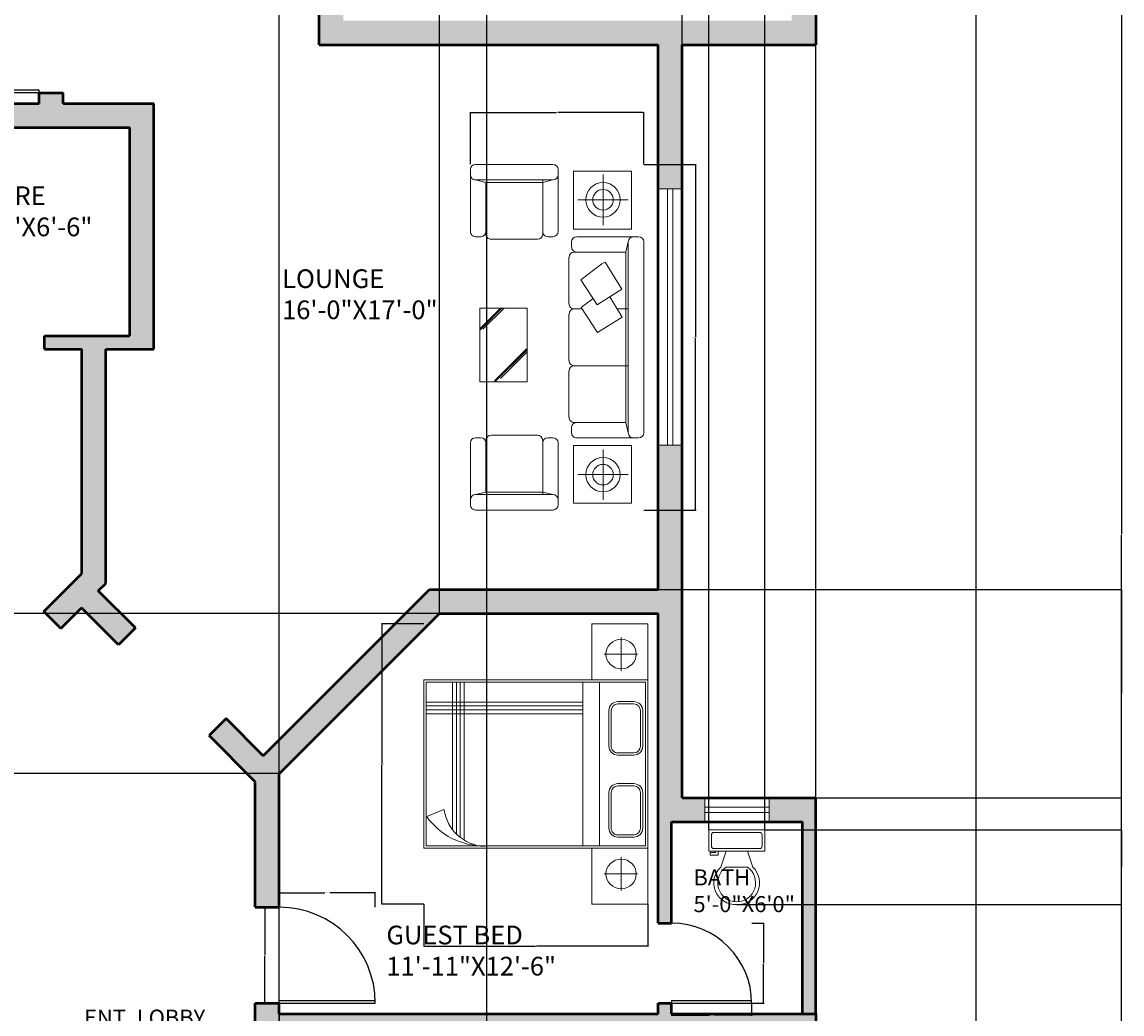
# Model space of a CAD drawing. Units: inches. Extents: x 134045 to 134755, y 144691 to 145880.
# Tile 5 of 6: x 134343 to 134755, y 145178 to 145550. Entities that reach past the tile are written whole.
import ezdxf

# ---------------------------------------------------------------- set-up
doc = ezdxf.new("R2010")
doc.units = ezdxf.units.IN
for name, color, linetype, lineweight in [('A-ANNO-DIMS', 2, 'Continuous', 18), ('A-AREA-IDEN', 7, 'Continuous', 18), ('A-DOOR', 4, 'Continuous', 25), ('A-FLOR-FIXT', 9, 'Continuous', 18), ('A-FURN', 8, 'Continuous', 18), ('A-GLAZ', 4, 'Continuous', 18), ('A-WALL', 7, 'Continuous', 50), ('A-WALL-PATT', 252, 'Continuous', 13), ('C-PROP', 7, 'Continuous', 25)]:
    doc.layers.add(name, color=color, linetype=linetype, lineweight=lineweight)
doc.styles.get("Standard").update_dxf_attribs({"font": 'arial.ttf'})
doc.dimstyles.get("Standard").update_dxf_attribs({"dimtxt": 0.18, "dimasz": 0.18, "dimexe": 0.18, "dimexo": 0.0625, "dimgap": 0.09, "dimtad": 0, "dimtih": 1, "dimtoh": 1, "dimdec": 4, "dimzin": 0, "dimdsep": 46, "dimtxsty": 'Standard', "dimcen": 0.09, "dimadec": 0, "dimazin": 0, "dimtfac": 1, "dimtdec": 4, "dimtofl": 0, "dimtmove": 0, "dimatfit": 3, "dimfxl": 1, "dimtolj": 1, "dimtzin": 0, "dimarcsym": 0})

# ---------------------------------------------------------------- blocks, each defined once
blk = doc.blocks.new('A$C780F33EA')
for p, q in [((687, 1011), (687, 1600)), ((726, 1649), (726, 1648)), ((2552, 1649), (736, 1649)), ((2601, 1011), (2601, 1600)), ((2601, 1600), (2601, 1551)), ((338, 1022), (338, 1500)), ((2552, 1502), (736, 1502)), ((736, 1502), (834, 1477)), ((2454, 1477), (834, 1477)), ((834, 1477), (834, 987)), ((1374, 1502), (1374, 1396)), ((1914, 1502), (1914, 987)), ((2552, 1502), (2454, 1477)), ((2454, 1477), (2454, 987)), ((2949, 1022), (2949, 1500)), ((576, 1264), (97, 1264)), ((2712, 1264), (3191, 1264)), ((1374, 1063), (1374, 987)), ((736, 962), (785, 962)), ((2552, 962), (2503, 962)), ((1325, 937), (883, 937)), ((1423, 937), (1865, 937)), ((2405, 937), (1963, 937)), ((0, 49), (0, 785)), ((638, 835), (49, 835)), ((147, 49), (147, 785)), ((147, 785), (172, 687)), ((687, 785), (687, 736)), ((2600, 785), (2600, 736)), ((2649, 835), (3238, 835)), ((3140, 785), (3116, 687)), ((3140, 49), (3140, 785)), ((3288, 49), (3288, 785)), ((147, 687), (663, 687)), ((172, 147), (172, 687)), ((172, 687), (663, 687)), ((656, 691), (656, 687)), ((712, 196), (712, 638)), ((2576, 196), (2576, 638)), ((3116, 687), (2625, 687)), ((3140, 687), (2625, 687)), ((2631, 691), (2631, 687)), ((3116, 147), (3116, 687)), ((2058, 230), (1754, 534)), ((2068, 232), (1765, 535)), ((2036, 285), (1782, 539)), ((1568, 118), (1368, 319)), ((1575, 89), (1368, 297)), ((1563, 89), (1368, 285)), ((147, 49), (172, 147)), ((172, 147), (663, 147)), ((656, 147), (656, 144)), ((3116, 147), (2625, 147)), ((2631, 147), (2631, 144)), ((3140, 49), (3116, 147)), ((638, 0), (49, 0)), ((49, 0), (98, 0)), ((687, 49), (687, 98)), ((2600, 49), (2600, 98)), ((2649, 0), (3238, 0)), ((3238, 0), (3189, 0))]:
    blk.add_line(p, q)
for points in [[(615, 1531), (65, 1531), (65, 981), (615, 981)], [(2672, 1531), (3222, 1531), (3222, 981), (2672, 981)], [(946, 1249), (1096, 1051), (1336, 1206), (1187, 1440), (928, 1281)], [(1368, 539), (2068, 539), (2068, 89), (1368, 89)]]:
    blk.add_lwpolyline(points, close=True)
blk.add_lwpolyline([(1275, 1166), (1360, 1054), (1600, 1209), (1451, 1443), (1260, 1325)])
for centre, radius in [((336, 1261), 164), ((2951, 1261), 164), ((336, 1261), 97.9), ((2951, 1261), 97.9)]:
    blk.add_circle(centre, radius)
for centre, start, end in [((736, 1600), 90, 180), ((2552, 1600), 0, 90), ((2552, 1600), 0, 90), ((736, 1551), 180, 270), ((2552, 1551), 270, 0), ((736, 1011), 180, 270), ((785, 1011), 270, 0), ((883, 987), 180, 270), ((1325, 987), 270, 0), ((1423, 987), 180, 270), ((1865, 987), 270, 0), ((1963, 987), 180, 270), ((2405, 987), 270, 0), ((2503, 1011), 180, 270), ((2552, 1011), 270, 0), ((49, 785), 90, 180), ((98, 785), 0, 90), ((638, 785), 0, 90), ((638, 736), 270, 0), ((2649, 785), 90, 180), ((2649, 736), 180, 270), ((3189, 785), 90, 180), ((3238, 785), 0, 90), ((663, 638), 0, 90), ((2625, 638), 90, 180), ((638, 98), 0, 90), ((663, 196), 270, 0), ((2625, 196), 180, 270), ((2649, 98), 90, 180), ((49, 49), 180, 270), ((49, 49), 180, 270), ((98, 49), 270, 0), ((638, 49), 270, 0), ((2649, 49), 180, 270), ((3189, 49), 180, 270), ((3238, 49), 270, 0), ((3238, 49), 270, 0)]:
    blk.add_arc(centre, 49.1, start, end)
blk = doc.blocks.new('A$C057D194F')
for p, q in [((0, 1.5, -0.1688), (0, 2, -0.1688)), ((0, 2, -0.1688), (0.5, 2, -0.1688)), ((0.5, 2, -0.1688), (0.5, 0, -0.1688)), ((2, 2, -0.1688), (0.5, 2, -0.1688)), ((1.98, 1.98, -0.1688), (0.52, 1.98, -0.1688)), ((0.52, 1.98, -0.1688), (0.52, 0.02, -0.1688)), ((1.98, 0.02, -0.1688), (1.98, 1.98, -0.1688)), ((2, 0, -0.1688), (2, 2, -0.1688)), ((2.5, 2, -0.1688), (2, 2, -0.1688)), ((2.5, 1.5, -0.1688), (2.5, 2, -0.1688)), ((0.2687, 1.9081, -0.1688), (0.2687, 1.761, -0.1688)), ((0.2687, 1.6081, -0.1688), (0.2687, 1.9081, -0.1688)), ((0.6935, 1.8739, -0.1688), (0.6935, 1.7322, -0.1688)), ((0.7135, 1.8739, -0.1688), (0.7135, 1.7322, -0.1688)), ((1.0907, 1.9539, -0.1688), (0.7735, 1.9539, -0.1688)), ((1.0907, 1.9339, -0.1688), (0.7735, 1.9339, -0.1688)), ((1.1507, 1.7322, -0.1688), (1.1507, 1.8739, -0.1688)), ((1.1707, 1.7322, -0.1688), (1.1707, 1.8739, -0.1688)), ((1.4252, 1.8739, -0.1688), (1.4252, 1.7322, -0.1688)), ((1.4452, 1.8739, -0.1688), (1.4452, 1.7322, -0.1688)), ((1.8224, 1.9539, -0.1688), (1.5052, 1.9539, -0.1688)), ((1.8224, 1.9339, -0.1688), (1.5052, 1.9339, -0.1688)), ((1.8824, 1.7322, -0.1688), (1.8824, 1.8739, -0.1688)), ((1.9024, 1.7322, -0.1688), (1.9024, 1.8739, -0.1688)), ((2.2313, 1.9081, -0.1688), (2.2313, 1.761, -0.1688)), ((2.2313, 1.6081, -0.1688), (2.2313, 1.9081, -0.1688)), ((0.4194, 1.761, -0.1688), (0.1194, 1.761, -0.1688)), ((0.2687, 1.761, -0.1688), (0.4194, 1.761, -0.1688)), ((0.2687, 1.761, -0.1688), (0.2687, 1.6081, -0.1688)), ((0.7735, 1.6722, -0.1688), (1.0907, 1.6722, -0.1688)), ((1.5052, 1.6722, -0.1688), (1.8224, 1.6722, -0.1688)), ((2.0806, 1.761, -0.1688), (2.3806, 1.761, -0.1688)), ((2.2313, 1.761, -0.1688), (2.0806, 1.761, -0.1688)), ((2.2313, 1.761, -0.1688), (2.2313, 1.6081, -0.1688)), ((0.7735, 1.6522, -0.1688), (1.0907, 1.6522, -0.1688)), ((1.5052, 1.6522, -0.1688), (1.8224, 1.6522, -0.1688)), ((0.5, 1.5, -0.1688), (0, 1.5, -0.1688)), ((1.98, 1.5693, -0.1688), (0.52, 1.5693, -0.1688)), ((2, 1.5, -0.1688), (2.5, 1.5, -0.1688)), ((1.98, 1.4193, -0.1688), (0.52, 1.4193, -0.1688)), ((0.6969, 0.02, -0.1688), (0.6969, 1.4193, -0.1688)), ((0.7319, 0.02, -0.1688), (0.7319, 1.4193, -0.1688)), ((0.7669, 0.02, -0.1688), (0.7669, 1.4193, -0.1688)), ((0.8019, 0.02, -0.1688), (0.8019, 1.4193, -0.1688)), ((0.52, 0.3595, -0.1688), (1.9292, 0.3595, -0.1688)), ((0.52, 0.3245, -0.1688), (1.905, 0.3245, -0.1688)), ((0.52, 0.2895, -0.1688), (1.8742, 0.2895, -0.1688)), ((0.52, 0.2545, -0.1688), (1.8344, 0.2545, -0.1688)), ((1.6548, 0.1789, -0.1688), (1.7198, 0.0251, -0.1688)), ((0.52, 0.02, -0.1688), (1.98, 0.02, -0.1688)), ((0.5, 0, -0.1688), (2, 0, -0.1688))]:
    blk.add_line(p, q)
for centre, radius, start, end in [((0.7735, 1.8739, -0.1688), 0.08, 90, 180), ((0.7735, 1.8739, -0.1688), 0.06, 90, 180), ((1.0907, 1.8739, -0.1688), 0.08, 0, 90), ((1.0907, 1.8739, -0.1688), 0.06, 0, 90), ((1.5052, 1.8739, -0.1688), 0.08, 90, 180), ((1.5052, 1.8739, -0.1688), 0.06, 90, 180), ((1.8224, 1.8739, -0.1688), 0.08, 0, 90), ((1.8224, 1.8739, -0.1688), 0.06, 0, 90), ((0.7735, 1.7322, -0.1688), 0.08, 180, 270), ((0.7735, 1.7322, -0.1688), 0.06, 180, 270), ((1.0907, 1.7322, -0.1688), 0.08, 270, 0), ((1.0907, 1.7322, -0.1688), 0.06, 270, 0), ((1.5052, 1.7322, -0.1688), 0.08, 180, 270), ((1.5052, 1.7322, -0.1688), 0.06, 180, 270), ((1.8224, 1.7322, -0.1688), 0.08, 270, 0), ((1.8224, 1.7322, -0.1688), 0.06, 270, 0), ((1.5992, 0.5623, -0.1688), 0.3874, 278.2518, 356.6808), ((1.363, 0.5286, -0.1688), 0.6171, 305.32946, 1.04595)]:
    blk.add_arc(centre, radius, start, end)
blk.add_ellipse((0.2687, 1.761, -0.1688), major_axis=(0, -0.1351), ratio=0.975448)
at = {"extrusion": (0, 0, -1)}
blk.add_ellipse((2.2313, 1.761, -0.1688), major_axis=(0, 0.1351), ratio=0.975448, dxfattribs=at)
for p in [(0.2687, 1.761, -0.1688), (2.2313, 1.761, -0.1688)]:
    blk.add_point(p)
blk = doc.blocks.new('*U7')
for p, q in [((9.5, -6), (9.5, -2)), ((-8, -8.5), (-8, -8)), ((-7, -8), (-7, -9.5)), ((-4, -8), (-6, -14)), ((4, -8), (6, -14)), ((-10, -8.5), (-8, -8.5)), ((-10, -9.5), (-10, -8.5)), ((-7, -9.5), (-10, -9.5)), ((4, -14), (-4, -14))]:
    blk.add_line(p, q)
blk.add_lwpolyline([(10.5, -8), (10.5, 0), (-10.5, 0), (-10.5, -8)], close=True)
for points in [[(-9.5, -2), (-9.5, -6)], [(8.5, -1), (-8.5, -1)], [(-8.5, -7), (8.5, -7)]]:
    blk.add_lwpolyline(points)
for centre, radius, start, end in [((-8.625, -1.875), 0.8839, 81.8699, 188.1301), ((8.625, -1.875), 0.8839, 351.8699, 98.1301), ((-8.625, -6.125), 0.8839, 171.869898, 278.1301), ((8.625, -6.125), 0.8839, 261.8699, 8.1301), ((-0.4772, -19.9188), 8.0953, 133.01722, 273.38), ((0.0374, -19.8731), 7.127, 124.50543, 269.7), ((-0.0373, -19.8731), 7.127, 270.3, 55.4946), ((0.4773, -19.9188), 8.0953, 266.62, 46.9828)]:
    blk.add_arc(centre, radius, start, end)
blk = doc.blocks.new('DOOR-SWING-36IN')
for p, q in [((0, 1), (35.99, 1)), ((0, 0), (0, 1)), ((0, 0), (36, 0))]:
    blk.add_line(p, q)
blk.add_arc((0, 0), 36, 0, 90)
blk = doc.blocks.new('DOOR-SWING-30IN')
for p, q in [((0, 1), (29.98, 1)), ((0, 1), (0, 0)), ((0, 0), (30, 0))]:
    blk.add_line(p, q)
blk.add_arc((0, 0), 30, 0, 90)
blk = doc.blocks.new('WIN-GLAZ-24IN')
for p, q in [((0, 0), (0, 24)), ((2, 0), (2, 24))]:
    blk.add_line(p, q)
blk = doc.blocks.new('WIN-GLAZ-96IN')
for p, q in [((0, 0), (0, 96)), ((2, 0), (2, 96))]:
    blk.add_line(p, q)
blk = doc.blocks.new('*D20')
at = {"layer": 'A-ANNO-DIMS', "color": 0, "lineweight": -2, "transparency": 16777216}
for p, q in [((134439.1, 145218.44), (134439.1, 145223.96)), ((134439.28, 145223.78), (134456.17, 145223.78)), ((134474.92, 145223.78), (134458.04, 145223.78)), ((134475.1, 145218.44), (134475.1, 145223.96))]:
    blk.add_line(p, q, dxfattribs=at)
at = {"layer": 'A-ANNO-DIMS', "color": 0, "transparency": 16777216}
for points in [[(134439.28, 145223.81), (134439.28, 145223.75), (134439.1, 145223.78)], [(134474.92, 145223.81), (134474.92, 145223.75), (134475.1, 145223.78)]]:
    blk.add_solid(points, dxfattribs=at)
at = {"layer": 'Defpoints', "color": 0, "transparency": 16777216}
for p in [(134475.1, 145223.78), (134439.1, 145218.38), (134475.1, 145218.38)]:
    blk.add_point(p, dxfattribs=at)
at = {"layer": 'A-ANNO-DIMS', "color": 0, "transparency": 16777216, "insert": (134457.1, 145223.78), "char_height": 0.18, "attachment_point": 5}
blk.add_mtext('\\A1;DOOR 36 TYP.', dxfattribs=at)
blk = doc.blocks.new('*D21')
at = {"layer": 'A-ANNO-DIMS', "color": 0, "lineweight": -2, "transparency": 16777216}
for p, q in [((134439.04, 145218.38), (134433.52, 145218.38)), ((134433.7, 145218.2), (134433.7, 145200.56)), ((134433.7, 145182.56), (134433.7, 145200.19)), ((134439.04, 145182.38), (134433.52, 145182.38))]:
    blk.add_line(p, q, dxfattribs=at)
at = {"layer": 'A-ANNO-DIMS', "color": 0, "transparency": 16777216}
for points in [[(134433.67, 145218.2), (134433.73, 145218.2), (134433.7, 145218.38)], [(134433.67, 145182.56), (134433.73, 145182.56), (134433.7, 145182.38)]]:
    blk.add_solid(points, dxfattribs=at)
at = {"layer": 'Defpoints', "color": 0, "transparency": 16777216}
for p in [(134433.7, 145218.38), (134439.1, 145218.38), (134439.1, 145182.38)]:
    blk.add_point(p, dxfattribs=at)
at = {"layer": 'A-ANNO-DIMS', "color": 0, "transparency": 16777216, "insert": (134433.7, 145200.38), "char_height": 0.18, "attachment_point": 5}
blk.add_mtext('\\A1;36 TYP.', dxfattribs=at)
blk = doc.blocks.new('*D22')
at = {"layer": 'A-ANNO-DIMS', "color": 0, "lineweight": -2, "transparency": 16777216}
for p, q in [((134586.1, 145182.31), (134586.1, 145177.7)), ((134616.1, 145182.31), (134616.1, 145177.7)), ((134586.28, 145177.88), (134600.17, 145177.88)), ((134615.92, 145177.88), (134602.04, 145177.88))]:
    blk.add_line(p, q, dxfattribs=at)
at = {"layer": 'A-ANNO-DIMS', "color": 0, "transparency": 16777216}
for points in [[(134586.28, 145177.91), (134586.28, 145177.85), (134586.1, 145177.88)], [(134615.92, 145177.91), (134615.92, 145177.85), (134616.1, 145177.88)]]:
    blk.add_solid(points, dxfattribs=at)
at = {"layer": 'Defpoints', "color": 0, "transparency": 16777216}
for p in [(134586.1, 145182.38), (134616.1, 145182.38), (134616.1, 145177.88)]:
    blk.add_point(p, dxfattribs=at)
at = {"layer": 'A-ANNO-DIMS', "color": 0, "transparency": 16777216, "insert": (134601.1, 145177.88), "char_height": 0.18, "attachment_point": 5}
blk.add_mtext('\\A1;DOOR 30 TYP.', dxfattribs=at)
blk = doc.blocks.new('*D23')
at = {"layer": 'A-ANNO-DIMS', "color": 0, "lineweight": -2, "transparency": 16777216}
for p, q in [((134616.17, 145212.38), (134620.78, 145212.38)), ((134620.6, 145212.2), (134620.6, 145197.56)), ((134620.6, 145182.56), (134620.6, 145197.19)), ((134616.17, 145182.38), (134620.78, 145182.38))]:
    blk.add_line(p, q, dxfattribs=at)
at = {"layer": 'A-ANNO-DIMS', "color": 0, "transparency": 16777216}
for points in [[(134620.57, 145212.2), (134620.63, 145212.2), (134620.6, 145212.38)], [(134620.57, 145182.56), (134620.63, 145182.56), (134620.6, 145182.38)]]:
    blk.add_solid(points, dxfattribs=at)
at = {"layer": 'Defpoints', "color": 0, "transparency": 16777216}
for p in [(134616.1, 145212.38), (134620.6, 145212.38), (134616.1, 145182.38)]:
    blk.add_point(p, dxfattribs=at)
at = {"layer": 'A-ANNO-DIMS', "color": 0, "transparency": 16777216, "insert": (134620.6, 145197.38), "char_height": 0.18, "attachment_point": 5}
blk.add_mtext('\\A1;30 TYP.', dxfattribs=at)
blk = doc.blocks.new('*D34')
at = {"layer": 'A-ANNO-DIMS', "color": 0, "lineweight": -2, "transparency": 16777216}
for p, q in [((134575.76, 145496.53), (134595.29, 145496.53)), ((134595.11, 145496.35), (134595.11, 145431.99)), ((134595.11, 145367.27), (134595.11, 145431.63)), ((134575.76, 145367.09), (134595.29, 145367.09))]:
    blk.add_line(p, q, dxfattribs=at)
at = {"layer": 'A-ANNO-DIMS', "color": 0, "transparency": 16777216}
for points in [[(134595.08, 145496.35), (134595.14, 145496.35), (134595.11, 145496.53)], [(134595.08, 145367.27), (134595.14, 145367.27), (134595.11, 145367.09)]]:
    blk.add_solid(points, dxfattribs=at)
at = {"layer": 'Defpoints', "color": 0, "transparency": 16777216}
for p in [(134575.7, 145496.53), (134575.7, 145367.09), (134595.11, 145367.09)]:
    blk.add_point(p, dxfattribs=at)
at = {"layer": 'A-ANNO-DIMS', "color": 0, "transparency": 16777216, "insert": (134595.11, 145431.81), "char_height": 0.18, "attachment_point": 5}
blk.add_mtext('\\A1;LOUNGE SET 129', dxfattribs=at)
blk = doc.blocks.new('*D35')
at = {"layer": 'A-ANNO-DIMS', "color": 0, "lineweight": -2, "transparency": 16777216}
for p, q in [((134510.76, 145496.59), (134510.76, 145516.12)), ((134510.94, 145515.94), (134543.01, 145515.94)), ((134575.52, 145515.94), (134543.45, 145515.94)), ((134575.7, 145496.59), (134575.7, 145516.12))]:
    blk.add_line(p, q, dxfattribs=at)
at = {"layer": 'A-ANNO-DIMS', "color": 0, "transparency": 16777216}
for points in [[(134510.94, 145515.97), (134510.94, 145515.91), (134510.76, 145515.94)], [(134575.52, 145515.97), (134575.52, 145515.91), (134575.7, 145515.94)]]:
    blk.add_solid(points, dxfattribs=at)
at = {"layer": 'Defpoints', "color": 0, "transparency": 16777216}
for p in [(134575.7, 145515.94), (134510.76, 145496.53), (134575.7, 145496.53)]:
    blk.add_point(p, dxfattribs=at)
at = {"layer": 'A-ANNO-DIMS', "color": 0, "transparency": 16777216, "insert": (134543.23, 145515.94), "char_height": 0.18, "attachment_point": 5}
blk.add_mtext('\\A1;65', dxfattribs=at)
blk = doc.blocks.new('*D36')
at = {"layer": 'A-ANNO-DIMS', "color": 0, "lineweight": -2, "transparency": 16777216}
for p, q in [((134493.26, 145324.44), (134477.41, 145324.44)), ((134477.59, 145324.26), (134477.59, 145272.18)), ((134477.59, 145219.74), (134477.59, 145271.81)), ((134493.26, 145219.56), (134477.41, 145219.56))]:
    blk.add_line(p, q, dxfattribs=at)
at = {"layer": 'A-ANNO-DIMS', "color": 0, "transparency": 16777216}
for points in [[(134477.56, 145324.26), (134477.62, 145324.26), (134477.59, 145324.44)], [(134477.56, 145219.74), (134477.62, 145219.74), (134477.59, 145219.56)]]:
    blk.add_solid(points, dxfattribs=at)
at = {"layer": 'Defpoints', "color": 0, "transparency": 16777216}
for p in [(134493.32, 145324.44), (134477.59, 145219.56), (134493.32, 145219.56)]:
    blk.add_point(p, dxfattribs=at)
at = {"layer": 'A-ANNO-DIMS', "color": 0, "transparency": 16777216, "insert": (134477.59, 145272), "char_height": 0.18, "attachment_point": 5}
blk.add_mtext('\\A1;BED GROUP 105', dxfattribs=at)
blk = doc.blocks.new('*D37')
at = {"layer": 'A-ANNO-DIMS', "color": 0, "lineweight": -2, "transparency": 16777216}
for p, q in [((134493.32, 145219.49), (134493.32, 145203.64)), ((134577.23, 145219.49), (134577.23, 145203.64)), ((134493.5, 145203.82), (134535.06, 145203.82)), ((134577.05, 145203.82), (134535.49, 145203.82))]:
    blk.add_line(p, q, dxfattribs=at)
at = {"layer": 'A-ANNO-DIMS', "color": 0, "transparency": 16777216}
for points in [[(134493.5, 145203.85), (134493.5, 145203.79), (134493.32, 145203.82)], [(134577.05, 145203.85), (134577.05, 145203.79), (134577.23, 145203.82)]]:
    blk.add_solid(points, dxfattribs=at)
at = {"layer": 'Defpoints', "color": 0, "transparency": 16777216}
for p in [(134493.32, 145219.56), (134577.23, 145219.56), (134577.23, 145203.82)]:
    blk.add_point(p, dxfattribs=at)
at = {"layer": 'A-ANNO-DIMS', "color": 0, "transparency": 16777216, "insert": (134535.28, 145203.82), "char_height": 0.18, "attachment_point": 5}
blk.add_mtext('\\A1;84', dxfattribs=at)
blk = doc.blocks.new('*D49')
at = {"layer": 'A-ANNO-DIMS', "color": 0, "lineweight": -2, "transparency": 16777216}
for p, q in [((134640.17, 145765.38), (134754.83, 145765.38)), ((134754.65, 145765.2), (134754.65, 145358.06)), ((134754.65, 144950.56), (134754.65, 145357.69)), ((134640.17, 144950.38), (134754.83, 144950.38))]:
    blk.add_line(p, q, dxfattribs=at)
at = {"layer": 'A-ANNO-DIMS', "color": 0, "transparency": 16777216}
for points in [[(134754.62, 145765.2), (134754.68, 145765.2), (134754.65, 145765.38)], [(134754.62, 144950.56), (134754.68, 144950.56), (134754.65, 144950.38)]]:
    blk.add_solid(points, dxfattribs=at)
at = {"layer": 'Defpoints', "color": 0, "transparency": 16777216}
for p in [(134640.1, 145765.38), (134754.65, 145765.38), (134640.1, 144950.38)]:
    blk.add_point(p, dxfattribs=at)
at = {"layer": 'A-ANNO-DIMS', "color": 0, "transparency": 16777216, "insert": (134754.65, 145357.88), "char_height": 0.18, "attachment_point": 5}
blk.add_mtext('\\A1;815', dxfattribs=at)
blk = doc.blocks.new('*D57')
at = {"layer": 'A-ANNO-DIMS', "color": 0, "lineweight": -2, "transparency": 16777216}
for p, q in [((134590.1, 145259.44), (134590.1, 145880.11)), ((134590.28, 145879.93), (134614.89, 145879.93)), ((134639.92, 145879.93), (134615.32, 145879.93)), ((134640.1, 145259.44), (134640.1, 145880.11))]:
    blk.add_line(p, q, dxfattribs=at)
at = {"layer": 'A-ANNO-DIMS', "color": 0, "transparency": 16777216}
for points in [[(134590.28, 145879.96), (134590.28, 145879.9), (134590.1, 145879.93)], [(134639.92, 145879.96), (134639.92, 145879.9), (134640.1, 145879.93)]]:
    blk.add_solid(points, dxfattribs=at)
at = {"layer": 'Defpoints', "color": 0, "transparency": 16777216}
for p in [(134590.1, 145879.93), (134590.1, 145259.38), (134640.1, 145259.38)]:
    blk.add_point(p, dxfattribs=at)
at = {"layer": 'A-ANNO-DIMS', "color": 0, "transparency": 16777216, "insert": (134615.1, 145879.93), "char_height": 0.18, "attachment_point": 5}
blk.add_mtext('\\A1;50', dxfattribs=at)
blk = doc.blocks.new('*D58')
at = {"layer": 'A-ANNO-DIMS', "color": 0, "lineweight": -2, "transparency": 16777216}
for p, q in [((134600.01, 145247.44), (134600.01, 145880.11)), ((134600.19, 145879.93), (134610.3, 145879.93)), ((134620.83, 145879.93), (134610.71, 145879.93)), ((134621.01, 145247.44), (134621.01, 145880.11))]:
    blk.add_line(p, q, dxfattribs=at)
at = {"layer": 'A-ANNO-DIMS', "color": 0, "transparency": 16777216}
for points in [[(134600.19, 145879.96), (134600.19, 145879.9), (134600.01, 145879.93)], [(134620.83, 145879.96), (134620.83, 145879.9), (134621.01, 145879.93)]]:
    blk.add_solid(points, dxfattribs=at)
at = {"layer": 'Defpoints', "color": 0, "transparency": 16777216}
for p in [(134621.01, 145879.93), (134600.01, 145247.37), (134621.01, 145247.37)]:
    blk.add_point(p, dxfattribs=at)
at = {"layer": 'A-ANNO-DIMS', "color": 0, "transparency": 16777216, "insert": (134610.51, 145879.93), "char_height": 0.18, "attachment_point": 5}
blk.add_mtext('\\A1;21', dxfattribs=at)
blk = doc.blocks.new('*D59')
at = {"layer": 'A-ANNO-DIMS', "color": 0, "lineweight": -2, "transparency": 16777216}
for p, q in [((134621.07, 145247.37), (134754.83, 145247.37)), ((134754.65, 145247.19), (134754.65, 145233.55)), ((134754.65, 145219.55), (134754.65, 145233.19)), ((134610.57, 145219.37), (134754.83, 145219.37))]:
    blk.add_line(p, q, dxfattribs=at)
at = {"layer": 'A-ANNO-DIMS', "color": 0, "transparency": 16777216}
for points in [[(134754.62, 145247.19), (134754.68, 145247.19), (134754.65, 145247.37)], [(134754.62, 145219.55), (134754.68, 145219.55), (134754.65, 145219.37)]]:
    blk.add_solid(points, dxfattribs=at)
at = {"layer": 'Defpoints', "color": 0, "transparency": 16777216}
for p in [(134621.01, 145247.37), (134754.65, 145247.37), (134610.51, 145219.37)]:
    blk.add_point(p, dxfattribs=at)
at = {"layer": 'A-ANNO-DIMS', "color": 0, "transparency": 16777216, "insert": (134754.65, 145233.37), "char_height": 0.18, "attachment_point": 5}
blk.add_mtext('\\A1;28', dxfattribs=at)
blk = doc.blocks.new('*D60')
at = {"layer": 'A-ANNO-DIMS', "color": 0, "lineweight": -2, "transparency": 16777216}
for p, q in [((134439.1, 145268.44), (134439.1, 145880.11)), ((134439.28, 145879.93), (134468.88, 145879.93)), ((134498.92, 145879.93), (134469.32, 145879.93)), ((134499.1, 145328.44), (134499.1, 145880.11))]:
    blk.add_line(p, q, dxfattribs=at)
at = {"layer": 'A-ANNO-DIMS', "color": 0, "transparency": 16777216}
for points in [[(134439.28, 145879.96), (134439.28, 145879.9), (134439.1, 145879.93)], [(134498.92, 145879.96), (134498.92, 145879.9), (134499.1, 145879.93)]]:
    blk.add_solid(points, dxfattribs=at)
at = {"layer": 'Defpoints', "color": 0, "transparency": 16777216}
for p in [(134499.1, 145879.93), (134499.1, 145328.38), (134439.1, 145268.38)]:
    blk.add_point(p, dxfattribs=at)
at = {"layer": 'A-ANNO-DIMS', "color": 0, "transparency": 16777216, "insert": (134469.1, 145879.93), "char_height": 0.18, "attachment_point": 5}
blk.add_mtext('\\A1;60', dxfattribs=at)
blk = doc.blocks.new('*D61')
at = {"layer": 'A-ANNO-DIMS', "color": 0, "lineweight": -2, "transparency": 16777216}
for p, q in [((134499.04, 145328.38), (134045.37, 145328.38)), ((134045.55, 145328.2), (134045.55, 145298.56)), ((134045.55, 145268.56), (134045.55, 145298.19)), ((134439.04, 145268.38), (134045.37, 145268.38))]:
    blk.add_line(p, q, dxfattribs=at)
at = {"layer": 'A-ANNO-DIMS', "color": 0, "transparency": 16777216}
for points in [[(134045.52, 145328.2), (134045.58, 145328.2), (134045.55, 145328.38)], [(134045.52, 145268.56), (134045.58, 145268.56), (134045.55, 145268.38)]]:
    blk.add_solid(points, dxfattribs=at)
at = {"layer": 'Defpoints', "color": 0, "transparency": 16777216}
for p in [(134045.55, 145328.38), (134499.1, 145328.38), (134439.1, 145268.38)]:
    blk.add_point(p, dxfattribs=at)
at = {"layer": 'A-ANNO-DIMS', "color": 0, "transparency": 16777216, "insert": (134045.55, 145298.38), "char_height": 0.18, "attachment_point": 5}
blk.add_mtext('\\A1;60', dxfattribs=at)
blk = doc.blocks.new('*D64')
at = {"layer": 'A-ANNO-DIMS', "color": 0, "lineweight": -2, "transparency": 16777216}
for p, q in [((134430.1, 145182.31), (134430.1, 144690.65)), ((134439.1, 145178.31), (134439.1, 144690.65)), ((134430.28, 144690.83), (134434.45, 144690.83)), ((134438.92, 144690.83), (134434.75, 144690.83))]:
    blk.add_line(p, q, dxfattribs=at)
at = {"layer": 'A-ANNO-DIMS', "color": 0, "transparency": 16777216}
for points in [[(134430.28, 144690.86), (134430.28, 144690.8), (134430.1, 144690.83)], [(134438.92, 144690.86), (134438.92, 144690.8), (134439.1, 144690.83)]]:
    blk.add_solid(points, dxfattribs=at)
at = {"layer": 'Defpoints', "color": 0, "transparency": 16777216}
for p in [(134430.1, 145182.38), (134439.1, 145178.38), (134439.1, 144690.83)]:
    blk.add_point(p, dxfattribs=at)
at = {"layer": 'A-ANNO-DIMS', "color": 0, "transparency": 16777216, "insert": (134434.6, 144690.83), "char_height": 0.18, "attachment_point": 5}
blk.add_mtext('\\A1;9', dxfattribs=at)
blk = doc.blocks.new('*D66')
at = {"layer": 'A-ANNO-DIMS', "color": 0, "lineweight": -2, "transparency": 16777216}
for p, q in [((134439.1, 144959.44), (134439.1, 145880.11)), ((134439.28, 145879.93), (134477.68, 145879.93)), ((134516.72, 145879.93), (134478.32, 145879.93)), ((134516.9, 144959.44), (134516.9, 145880.11))]:
    blk.add_line(p, q, dxfattribs=at)
at = {"layer": 'A-ANNO-DIMS', "color": 0, "transparency": 16777216}
for points in [[(134439.28, 145879.96), (134439.28, 145879.9), (134439.1, 145879.93)], [(134516.72, 145879.96), (134516.72, 145879.9), (134516.9, 145879.93)]]:
    blk.add_solid(points, dxfattribs=at)
at = {"layer": 'Defpoints', "color": 0, "transparency": 16777216}
for p in [(134516.9, 145879.93), (134439.1, 144959.38), (134516.9, 144959.38)]:
    blk.add_point(p, dxfattribs=at)
at = {"layer": 'A-ANNO-DIMS', "color": 0, "transparency": 16777216, "insert": (134478, 145879.93), "char_height": 0.18, "attachment_point": 5}
blk.add_mtext('\\A1;77.8', dxfattribs=at)
blk = doc.blocks.new('*D68')
at = {"layer": 'A-ANNO-DIMS', "color": 0, "lineweight": -2, "transparency": 16777216}
for p, q in [((134581.17, 145337.38), (134754.83, 145337.38)), ((134754.65, 145337.2), (134754.65, 145298.56)), ((134754.65, 145259.56), (134754.65, 145298.19)), ((134590.17, 145259.38), (134754.83, 145259.38))]:
    blk.add_line(p, q, dxfattribs=at)
at = {"layer": 'A-ANNO-DIMS', "color": 0, "transparency": 16777216}
for points in [[(134754.62, 145337.2), (134754.68, 145337.2), (134754.65, 145337.38)], [(134754.62, 145259.56), (134754.68, 145259.56), (134754.65, 145259.38)]]:
    blk.add_solid(points, dxfattribs=at)
at = {"layer": 'Defpoints', "color": 0, "transparency": 16777216}
for p in [(134581.1, 145337.38), (134754.65, 145337.38), (134590.1, 145259.38)]:
    blk.add_point(p, dxfattribs=at)
at = {"layer": 'A-ANNO-DIMS', "color": 0, "transparency": 16777216, "insert": (134754.65, 145298.38), "char_height": 0.18, "attachment_point": 5}
blk.add_mtext('\\A1;78', dxfattribs=at)

msp = doc.modelspace()

# ---------------------------------------------------------------- hatches: boundary and pattern name
at = {"layer": 'A-WALL-PATT'}
h = msp.add_hatch(color=256, dxfattribs=at)
h.dxf.hatch_style = 1
h.paths.add_polyline_path([(134640.1037, 145765.3753), (134583.1037, 145765.3753), (134583.1037, 145756.3753), (134631.1037, 145756.3753), (134631.1037, 145550.3753), (134463.1037, 145550.3753), (134463.1037, 145554.3753), (134454.1037, 145554.3753), (134454.1037, 145541.3753), (134581.1037, 145541.3753), (134581.1037, 145487.3753), (134590.1037, 145487.3753), (134590.1037, 145541.3753), (134640.1037, 145541.3753)])
h = msp.add_hatch(color=256, dxfattribs=at)
h.dxf.hatch_style = 1
h.paths.add_polyline_path([(134169.1037, 145427.3753), (134266.1037, 145427.3753), (134266.1037, 145432.3753), (134217.1037, 145432.3753), (134217.1037, 145436.3753), (134208.1037, 145436.3753), (134208.1037, 145432.3753), (134160.1037, 145432.3753), (134160.1037, 145374.4227), (134169.1037, 145374.4227)], flags=17)
h.paths.add_polyline_path([(134217.1037, 145479.3753), (134208.1037, 145479.3753), (134208.1037, 145472.3753), (134217.1037, 145472.3753)], flags=17)
h.paths.add_polyline_path([(134217.1037, 145510.3753), (134306.1037, 145510.3753), (134306.1037, 145432.3753), (134302.1037, 145432.3753), (134302.1037, 145427.3753), (134315.1037, 145427.3753), (134315.1037, 145432.3753), (134311.1037, 145432.3753), (134311.1037, 145510.3753), (134383.1037, 145510.3753), (134383.1037, 145432.3753), (134351.1037, 145432.3753), (134351.1037, 145427.3753), (134365.1037, 145427.3753), (134365.1037, 145343.3753), (134350.8634, 145329.135), (134357.2273, 145322.771), (134364.9677, 145330.5114), (134378.8831, 145316.5959), (134385.2471, 145322.9598), (134371.3316, 145336.8753), (134374.1037, 145339.6474), (134374.1037, 145427.3753), (134392.1037, 145427.3753), (134392.1037, 145519.3753), (134358.1037, 145519.3753), (134358.1037, 145523.3753), (134349.1037, 145523.3753), (134349.1037, 145519.3753), (134169.1037, 145519.3753), (134169.1037, 145549.3753), (134160.1037, 145549.3753), (134160.1037, 145510.3753), (134208.1037, 145510.3753), (134208.1037, 145503.3753), (134217.1037, 145503.3753)])
h = msp.add_hatch(color=256, dxfattribs=at)
h.dxf.hatch_style = 1
h.paths.add_polyline_path([(134590.1037, 145391.3753), (134581.1037, 145391.3753), (134581.1037, 145337.3753), (134495.3758, 145337.3753), (134433.1037, 145275.1032), (134419.1882, 145289.0187), (134412.8243, 145282.6548), (134430.1037, 145265.3753), (134430.1037, 145218.3753), (134439.1037, 145218.3753), (134439.1037, 145268.3753), (134499.1037, 145328.3753), (134581.1037, 145328.3753), (134581.1037, 145212.3753), (134586.1037, 145212.3753), (134586.1037, 145250.3753), (134598.6037, 145250.3753), (134598.6037, 145259.3753), (134590.1037, 145259.3753)])
h = msp.add_hatch(color=256, dxfattribs=at)
h.dxf.hatch_style = 1
h.paths.add_polyline_path([(134640.1037, 145259.3753), (134622.6037, 145259.3753), (134622.6037, 145250.3753), (134635.1037, 145250.3753), (134635.1037, 145178.3753), (134640.1037, 145178.3753)])
h = msp.add_hatch(color=256, dxfattribs=at)
h.dxf.hatch_style = 1
h.paths.add_polyline_path([(134640.1037, 145178.3753), (134586.1037, 145178.3753), (134586.1037, 145182.3753), (134581.1037, 145182.3753), (134581.1037, 145178.3753), (134439.1037, 145178.3753), (134439.1037, 145182.3753), (134430.1037, 145182.3753), (134430.1037, 145165.3753), (134439.1037, 145165.3753), (134439.1037, 145169.3753), (134631.1037, 145169.3753), (134631.1037, 144959.3753), (134516.8973, 144959.3753), (134516.8973, 144950.3753), (134640.1037, 144950.3753)])
h.paths.add_polyline_path([(134439.1037, 145129.3753), (134430.1037, 145129.3753), (134430.1037, 145103.3753), (134423.1948, 145103.3753), (134423.1948, 145094.3753), (134430.1037, 145094.3753), (134430.1037, 145028.0394), (134439.1037, 145028.0394)])

# ---------------------------------------------------------------- linework, layer by layer
at = {"layer": 'A-GLAZ'}
for p, q in [((134581.1037, 145487.3753), (134590.1037, 145487.3753)), ((134581.1037, 145391.3753), (134590.1037, 145391.3753)), ((134598.6037, 145250.3753), (134598.6037, 145259.3753)), ((134622.6037, 145250.3753), (134622.6037, 145259.3753))]:
    msp.add_line(p, q, dxfattribs=at)
at = {"layer": 'A-WALL'}
for p, q in [((134640.1037, 145765.3753), (134640.1037, 145541.3753)), ((134454.1037, 145541.3753), (134454.1037, 145554.3753)), ((134454.1037, 145541.3753), (134581.1037, 145541.3753)), ((134581.1037, 145337.3753), (134581.1037, 145541.3753)), ((134590.1037, 145259.3753), (134590.1037, 145541.3753)), ((134590.1037, 145541.3753), (134640.1037, 145541.3753)), ((134349.1037, 145519.3753), (134349.1037, 145523.3753)), ((134349.1037, 145523.3753), (134358.1037, 145523.3753)), ((134358.1037, 145519.3753), (134358.1037, 145523.3753)), ((134169.1037, 145519.3753), (134349.1037, 145519.3753)), ((134358.1037, 145519.3753), (134392.1037, 145519.3753)), ((134392.1037, 145427.3753), (134392.1037, 145519.3753)), ((134311.1037, 145510.3753), (134383.1037, 145510.3753)), ((134383.1037, 145432.3753), (134383.1037, 145510.3753)), ((134351.1037, 145427.3753), (134351.1037, 145432.3753)), ((134351.1037, 145432.3753), (134383.1037, 145432.3753)), ((134351.1037, 145427.3753), (134365.1037, 145427.3753)), ((134365.1037, 145343.3753), (134365.1037, 145427.3753)), ((134374.1037, 145339.6474), (134374.1037, 145427.3753)), ((134374.1037, 145427.3753), (134392.1037, 145427.3753)), ((134350.8634, 145329.135), (134365.1037, 145343.3753)), ((134371.3316, 145336.8753), (134374.1037, 145339.6474)), ((134385.2471, 145322.9598), (134371.3316, 145336.8753)), ((134433.1037, 145275.1032), (134495.3758, 145337.3753)), ((134495.3758, 145337.3753), (134581.1037, 145337.3753)), ((134357.2273, 145322.771), (134350.8634, 145329.135)), ((134357.2273, 145322.771), (134364.9677, 145330.5114)), ((134378.8831, 145316.5959), (134364.9677, 145330.5114)), ((134439.1037, 145268.3753), (134499.1037, 145328.3753)), ((134499.1037, 145328.3753), (134581.1037, 145328.3753)), ((134581.1037, 145212.3753), (134581.1037, 145328.3753)), ((134385.2471, 145322.9598), (134378.8831, 145316.5959)), ((134419.1882, 145289.0187), (134412.8243, 145282.6548)), ((134433.1037, 145275.1032), (134419.1882, 145289.0187)), ((134430.1037, 145265.3753), (134412.8243, 145282.6548)), ((134439.1037, 145218.3753), (134439.1037, 145268.3753)), ((134430.1037, 145218.3753), (134430.1037, 145265.3753)), ((134590.1037, 145259.3753), (134640.1037, 145259.3753)), ((134640.1037, 145178.3753), (134640.1037, 145259.3753)), ((134586.1037, 145250.3753), (134635.1037, 145250.3753)), ((134586.1037, 145212.3753), (134586.1037, 145250.3753)), ((134635.1037, 145178.3753), (134635.1037, 145250.3753)), ((134430.1037, 145218.3753), (134439.1037, 145218.3753)), ((134581.1037, 145212.3753), (134586.1037, 145212.3753)), ((134430.1037, 145182.3753), (134439.1037, 145182.3753)), ((134430.1037, 145165.3753), (134430.1037, 145182.3753)), ((134439.1037, 145178.3753), (134439.1037, 145182.3753)), ((134581.1037, 145178.3753), (134581.1037, 145182.3753)), ((134581.1037, 145182.3753), (134586.1037, 145182.3753)), ((134586.1037, 145178.3753), (134586.1037, 145182.3753)), ((134439.1037, 145178.3753), (134581.1037, 145178.3753)), ((134586.1037, 145178.3753), (134640.1037, 145178.3753)), ((134640.1037, 145178.3753), (134640.1037, 144950.3753))]:
    msp.add_line(p, q, dxfattribs=at)
at = {"layer": 'C-PROP'}
msp.add_line((134700.1037, 145825.3753), (134700.1037, 144745.3753), dxfattribs=at)

# ---------------------------------------------------------------- block references
at = {"layer": 'A-DOOR', "extrusion": (0, 0, -1), "zscale": -1}
msp.add_blockref('DOOR-SWING-36IN', (-134349.1034, 145523.375), dxfattribs=at)
at = {"layer": 'A-DOOR'}
for name, p in [('DOOR-SWING-36IN', (134439.104, 145182.375)), ('DOOR-SWING-30IN', (134586.104, 145182.375))]:
    msp.add_blockref(name, p, dxfattribs=at)
at = {"layer": 'A-FLOR-FIXT'}
msp.add_blockref('*U7', (134610.5058, 145247.3728), dxfattribs=at)
at = {"layer": 'A-FURN', "rotation": 270}
for name, p, xscale, yscale, zscale in [('A$C780F33EA', (134510.7646, 145496.5263), 0.0393700787401575, 0.0393700787401575, 0.0393700787401575), ('A$C057D194F', (134493.3238, 145324.4362), 41.95231926620095, 41.95231926620095, 41.95231926620095)]:
    msp.add_blockref(name, p, dxfattribs=dict(at, xscale=xscale, yscale=yscale, zscale=zscale))
at = {"layer": 'A-GLAZ'}
msp.add_blockref('WIN-GLAZ-96IN', (134584.604, 145391.375), dxfattribs=at)
at = {"layer": 'A-GLAZ', "rotation": 270}
msp.add_blockref('WIN-GLAZ-24IN', (134598.6034, 145255.875), dxfattribs=at)

# ---------------------------------------------------------------- texts
at = {"layer": 'A-AREA-IDEN', "attachment_point": 1}
for s, width, insert, char_height in [('STORE\\P6\'-0"X6\'-6"', 40.020524, (134321.4449, 145488.3122), 7), ('LOUNGE\\P16\'-0"X17\'-0"', 66.184678, (134440.1886, 145457.2552), 7), ('BATH\\P5\'-0"X6\'0"', 18.935481, (134594.3133, 145232.5254), 6), ('GUEST BED\\P11\'-11"X12\'-6"', 74.6313, (134479.2525, 145211.4565), 7), ('ENT. LOBBY\\P7\'-9"X8\'-9"', 198.060459, (134366.0069, 145180.0217), 6)]:
    msp.add_mtext_dynamic_manual_height_columns(s, width=width, gutter_width=12.5, heights=[0], dxfattribs=dict(at, insert=insert, char_height=char_height))

# ---------------------------------------------------------------- dimensions: what is measured, and where the dimension line sits
at = {"layer": 'A-ANNO-DIMS'}
for base, p1, p2, override, picture, middle in [((134499.1037, 145879.9253), (134439.1037, 145268.3753), (134499.1037, 145328.3753), {"dimdec": 0, "dimlfac": 1, "dimrnd": 0, "dimzin": 0, "dimdsep": 46, "dimlunit": 2}, '*D60', (134469.1037, 145879.9253)), ((134516.8973, 145879.9253), (134439.1037, 144959.3753), (134516.8973, 144959.3753), {"dimdec": 1, "dimlfac": 1, "dimrnd": 0, "dimzin": 0, "dimdsep": 46, "dimlunit": 2}, '*D66', (134478.0005, 145879.9253)), ((134590.1037, 145879.9253), (134640.1037, 145259.3753), (134590.1037, 145259.3753), {"dimdec": 0, "dimlfac": 1, "dimrnd": 0, "dimzin": 0, "dimdsep": 46, "dimlunit": 2}, '*D57', (134615.1037, 145879.9253)), ((134621.0058, 145879.9253), (134600.0058, 145247.3728), (134621.0058, 145247.3728), {"dimdec": 0, "dimlfac": 1, "dimrnd": 0, "dimzin": 0, "dimdsep": 46, "dimlunit": 2}, '*D58', (134610.5058, 145879.9253)), ((134575.6951, 145515.9409), (134510.7646, 145496.5263), (134575.6951, 145496.5263), {"dimdec": 0, "dimlfac": 1, "dimrnd": 0, "dimzin": 0, "dimdsep": 46, "dimlunit": 2}, '*D35', (134543.2298, 145515.9409)), ((134577.2285, 145203.8233), (134493.3238, 145219.5554), (134577.2285, 145219.5554), {"dimdec": 0, "dimlfac": 1, "dimrnd": 0, "dimzin": 0, "dimdsep": 46, "dimlunit": 2}, '*D37', (134535.2762, 145203.8233)), ((134439.1037, 144690.8253), (134430.1037, 145182.3753), (134439.1037, 145178.3753), {"dimdec": 0, "dimlfac": 1, "dimrnd": 0, "dimzin": 0, "dimdsep": 46, "dimlunit": 2}, '*D64', (134434.6037, 144690.8253))]:
    dim = msp.add_linear_dim(base=base, p1=p1, p2=p2, dimstyle='Standard', override=override, dxfattribs=at)
    dim.commit()
    dim.dimension.update_dxf_attribs({"geometry": picture, "text_midpoint": middle})
for base, p1, p2, picture, middle in [((134754.6537, 145765.3753), (134640.1037, 144950.3753), (134640.1037, 145765.3753), '*D49', (134754.6537, 145357.8753)), ((134754.6537, 145337.3753), (134590.1037, 145259.3753), (134581.1037, 145337.3753), '*D68', (134754.6537, 145298.3753)), ((134045.5537, 145328.3753), (134439.1037, 145268.3753), (134499.1037, 145328.3753), '*D61', (134045.5537, 145298.3753)), ((134754.6537, 145247.3728), (134610.5059, 145219.3728), (134621.0058, 145247.3728), '*D59', (134754.6537, 145233.3728))]:
    dim = msp.add_linear_dim(base=base, p1=p1, p2=p2, angle=90, dimstyle='Standard', override={"dimdec": 0, "dimlfac": 1, "dimrnd": 0, "dimzin": 0, "dimdsep": 46, "dimlunit": 2}, dxfattribs=at)
    dim.commit()
    dim.dimension.update_dxf_attribs({"geometry": picture, "text_midpoint": middle})
for base, p1, p2, angle, text, picture, middle in [((134595.1098, 145367.095), (134575.6951, 145496.5263), (134575.6951, 145367.095), 270, 'LOUNGE SET <>', '*D34', (134595.1098, 145431.8106)), ((134477.5917, 145219.5554), (134493.3238, 145324.4362), (134493.3238, 145219.5554), 270, 'BED GROUP <>', '*D36', (134477.5917, 145271.9958)), ((134433.7037, 145218.3753), (134439.1037, 145182.3753), (134439.1037, 145218.3753), 90, '<> TYP.', '*D21', (134433.7037, 145200.3753)), ((134620.6037, 145212.3753), (134616.1037, 145182.3753), (134616.1037, 145212.3753), 90, '<> TYP.', '*D23', (134620.6037, 145197.3753))]:
    dim = msp.add_linear_dim(base=base, p1=p1, p2=p2, angle=angle, text=text, dimstyle='Standard', override={"dimdec": 0, "dimlfac": 1, "dimrnd": 0, "dimzin": 0, "dimdsep": 46, "dimlunit": 2}, dxfattribs=at)
    dim.commit()
    dim.dimension.update_dxf_attribs({"geometry": picture, "text_midpoint": middle})
for base, p1, p2, picture, middle in [((134475.1037, 145223.7753), (134439.1037, 145218.3753), (134475.1037, 145218.3753), '*D20', (134457.1037, 145223.7753)), ((134616.1037, 145177.8753), (134586.1037, 145182.3753), (134616.1037, 145182.3753), '*D22', (134601.1037, 145177.8753))]:
    dim = msp.add_linear_dim(base=base, p1=p1, p2=p2, text='DOOR <> TYP.', dimstyle='Standard', override={"dimdec": 0, "dimlfac": 1, "dimrnd": 0, "dimzin": 0, "dimdsep": 46, "dimlunit": 2}, dxfattribs=at)
    dim.commit()
    dim.dimension.update_dxf_attribs({"geometry": picture, "text_midpoint": middle})

doc.saveas('drawing.dxf')
